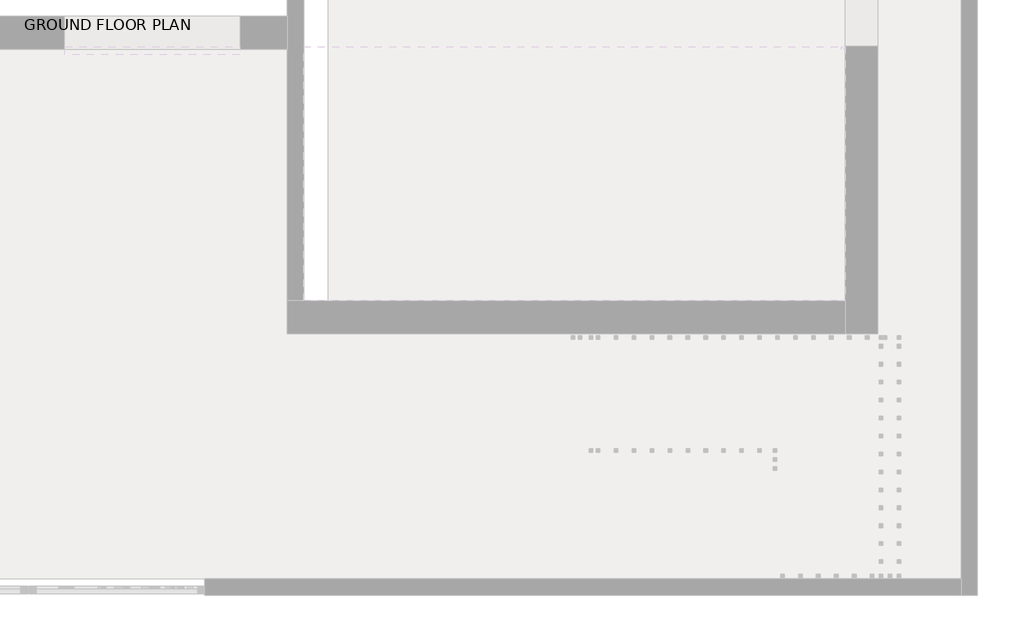
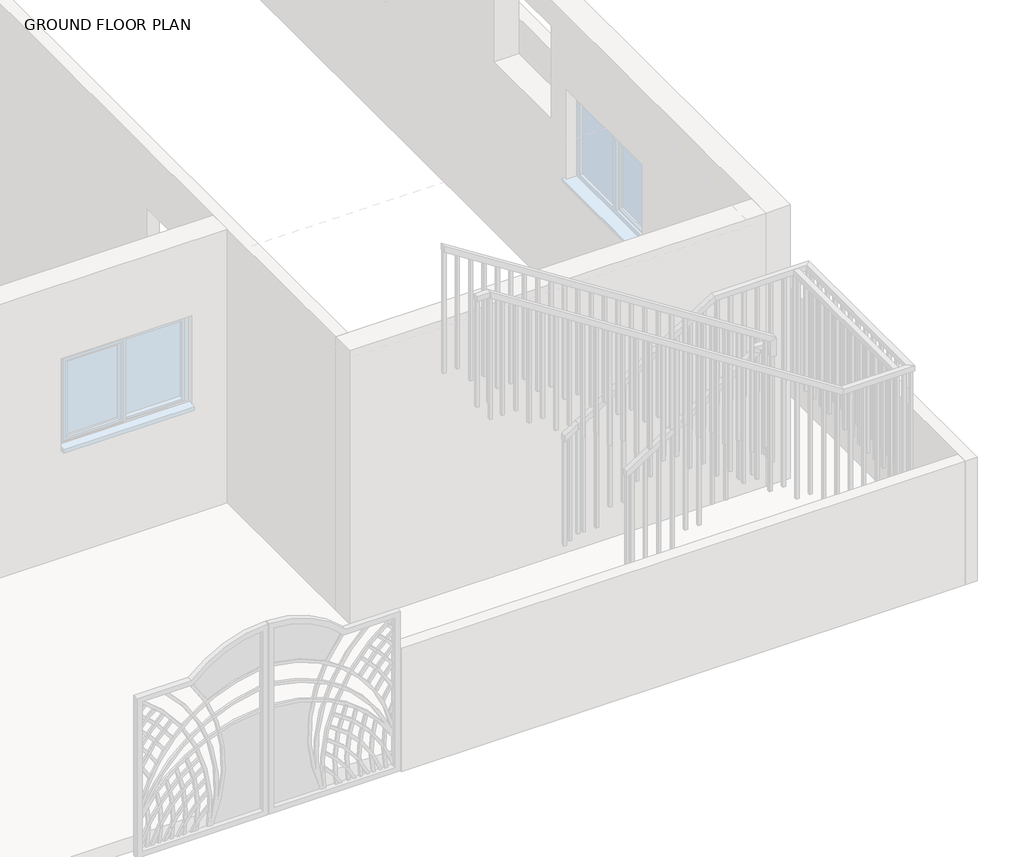
# One storey, part 7 of 23: 2 railings.
"""IFC4 building model written with IfcOpenShell, lengths in millimetres."""

from ifc_helpers import new_model, si_unit, frame, origin, place, context, project, spatial, polyline, outline, extrude, faceted_brep, element, save

model = new_model("IFC4")

# Units and contexts
model_context = context("Model", 3, world=origin())
ifc_project = project(units=[si_unit("LENGTHUNIT", "METRE", prefix="MILLI")], contexts=[model_context])

# Site, building, storey
site = spatial("IfcSite", under=ifc_project)
building = spatial("IfcBuilding", under=site)
storey = spatial("IfcBuildingStorey", under=building, Name="GROUND FLOOR PLAN", Elevation=487.68)

# Railings
placement = place(None, origin())
element("IfcRailing", 1, ObjectType="1100mm", at=placement, inside=storey, context=model_context, shape_type="SolidModel", body=[
    faceted_brep([(-8680.149573, -11007.9255223, 1912.8), (-8680.149573, -11007.9255223, 1853.4423995), (-8680.149573, -11057.9255223, 1853.4423995), (-8680.149573, -11057.9255223, 1912.8), (-7484.3306254, -11007.9255223, 2677.8717446), (-7434.3306254, -11007.9255223, 2650.5035914), (-7434.3306254, -11057.9255223, 2650.5035914), (-7484.3306254, -11057.9255223, 2677.8717446), (-7484.3306254, -11007.9255223, 2725.6), (-7434.3306254, -11007.9255223, 2675.6), (-7434.3306254, -11057.9255223, 2675.6), (-7484.3306254, -11057.9255223, 2725.6), (-7359.3306254, -11007.9255223, 2725.6), (-7359.3306254, -11007.9255223, 2675.6), (-7409.3306254, -11057.9255223, 2675.6), (-7409.3306254, -11057.9255223, 2725.6), (-7359.3306254, -11132.9255223, 2725.6), (-7359.3306254, -11132.9255223, 2675.6), (-7409.3306254, -11132.9255223, 2675.6), (-7409.3306254, -11132.9255223, 2725.6), (-7359.3306254, -11134.9255223, 2725.6), (-7409.3306254, -11134.9255223, 2725.6), (-7409.3306254, -11184.9255223, 2675.6), (-7359.3306254, -11184.9255223, 2675.6)], [[[0, 1, 2, 3]], [[1, 0, 4, 5]], [[2, 1, 5, 6]], [[3, 2, 6, 7]], [[0, 3, 7, 4]], [[5, 4, 8, 9]], [[6, 5, 9, 10]], [[7, 6, 10, 11]], [[4, 7, 11, 8]], [[9, 8, 12, 13]], [[10, 9, 13, 14]], [[11, 10, 14, 15]], [[8, 11, 15, 12]], [[13, 12, 16, 17]], [[14, 13, 17, 18]], [[15, 14, 18, 19]], [[12, 15, 19, 16]], [[20, 21, 22, 23]], [[17, 16, 20, 23]], [[18, 17, 23, 22]], [[19, 18, 22, 21]], [[16, 19, 21, 20]]]),
    faceted_brep([(-7359.3306254, -11184.9255223, 2855.9055527), (-7409.3306254, -11184.9255223, 2828.5415543), (-7409.3306254, -11134.9255223, 2828.5415543), (-7359.3306254, -11134.9255223, 2855.9055527), (-10457.8773536, -11184.9255223, 4838.88), (-10457.8773536, -11134.9255223, 4838.88), (-10457.8773536, -11134.9255223, 4779.517542), (-10457.8773536, -11184.9255223, 4779.517542)], [[[0, 1, 2, 3]], [[4, 5, 6, 7]], [[1, 0, 4, 7]], [[2, 1, 7, 6]], [[3, 2, 6, 5]], [[0, 3, 5, 4]]]),
    faceted_brep([(-7359.3306254, -11134.9255223, 2725.6), (-7359.3306254, -11184.9255223, 2675.6), (-7409.3306254, -11184.9255223, 2675.6), (-7409.3306254, -11134.9255223, 2725.6), (-7359.3306254, -11134.9255223, 2855.9055527), (-7409.3306254, -11134.9255223, 2828.5415543), (-7409.3306254, -11184.9255223, 2828.5415543), (-7359.3306254, -11184.9255223, 2855.9055527)], [[[0, 1, 2, 3]], [[4, 5, 6, 7]], [[1, 0, 4, 7]], [[2, 1, 7, 6]], [[3, 2, 6, 5]], [[0, 3, 5, 4]]]),
    extrude(outline(polyline([(3576.32, -10434.3306254), (4764.4483614, -10434.3306254), (4780.4475912, -10459.3306254), (3576.32, -10459.3306254), (3576.32, -10434.3306254)])), frame((0.0, -11172.4255223, 0.0), z_axis=(0.0, 1.0, 0.0), x_axis=(0.0, 0.0, 1.0)), (0.0, 0.0, 1.0), 25.0),
    extrude(outline(polyline([(3576.32, -10309.3306254), (4684.4522123, -10309.3306254), (4700.4514422, -10334.3306254), (3576.32, -10334.3306254), (3576.32, -10309.3306254)])), frame((0.0, -11172.4255223, 0.0), z_axis=(0.0, 1.0, 0.0), x_axis=(0.0, 0.0, 1.0)), (0.0, 0.0, 1.0), 25.0),
    extrude(outline(polyline([(3413.76, -10184.3306254), (4604.4560633, -10184.3306254), (4620.4552931, -10209.3306254), (3413.76, -10209.3306254), (3413.76, -10184.3306254)])), frame((0.0, -11172.4255223, 0.0), z_axis=(0.0, 1.0, 0.0), x_axis=(0.0, 0.0, 1.0)), (0.0, 0.0, 1.0), 25.0),
    extrude(outline(polyline([(3413.76, -10059.3306254), (4524.4599142, -10059.3306254), (4540.459144, -10084.3306254), (3413.76, -10084.3306254), (3413.76, -10059.3306254)])), frame((0.0, -11172.4255223, 0.0), z_axis=(0.0, 1.0, 0.0), x_axis=(0.0, 0.0, 1.0)), (0.0, 0.0, 1.0), 25.0),
    extrude(outline(polyline([(3251.2, -9934.3306254), (4444.4637652, -9934.3306254), (4460.462995, -9959.3306254), (3251.2, -9959.3306254), (3251.2, -9934.3306254)])), frame((0.0, -11172.4255223, 0.0), z_axis=(0.0, 1.0, 0.0), x_axis=(0.0, 0.0, 1.0)), (0.0, 0.0, 1.0), 25.0),
    extrude(outline(polyline([(3251.2, -9809.3306254), (4364.4676161, -9809.3306254), (4380.4668459, -9834.3306254), (3251.2, -9834.3306254), (3251.2, -9809.3306254)])), frame((0.0, -11172.4255223, 0.0), z_axis=(0.0, 1.0, 0.0), x_axis=(0.0, 0.0, 1.0)), (0.0, 0.0, 1.0), 25.0),
    extrude(outline(polyline([(3251.2, -9684.3306254), (4284.4714671, -9684.3306254), (4300.4706969, -9709.3306254), (3251.2, -9709.3306254), (3251.2, -9684.3306254)])), frame((0.0, -11172.4255223, 0.0), z_axis=(0.0, 1.0, 0.0), x_axis=(0.0, 0.0, 1.0)), (0.0, 0.0, 1.0), 25.0),
    extrude(outline(polyline([(3088.64, -9559.3306254), (4204.475318, -9559.3306254), (4220.4745478, -9584.3306254), (3088.64, -9584.3306254), (3088.64, -9559.3306254)])), frame((0.0, -11172.4255223, 0.0), z_axis=(0.0, 1.0, 0.0), x_axis=(0.0, 0.0, 1.0)), (0.0, 0.0, 1.0), 25.0),
    extrude(outline(polyline([(3088.64, -9434.3306254), (4124.479169, -9434.3306254), (4140.4783988, -9459.3306254), (3088.64, -9459.3306254), (3088.64, -9434.3306254)])), frame((0.0, -11172.4255223, 0.0), z_axis=(0.0, 1.0, 0.0), x_axis=(0.0, 0.0, 1.0)), (0.0, 0.0, 1.0), 25.0),
    extrude(outline(polyline([(2926.08, -9309.3306254), (4044.4830199, -9309.3306254), (4060.4822497, -9334.3306254), (2926.08, -9334.3306254), (2926.08, -9309.3306254)])), frame((0.0, -11172.4255223, 0.0), z_axis=(0.0, 1.0, 0.0), x_axis=(0.0, 0.0, 1.0)), (0.0, 0.0, 1.0), 25.0),
    extrude(outline(polyline([(2926.08, -9184.3306254), (3964.4868709, -9184.3306254), (3980.4861007, -9209.3306254), (2926.08, -9209.3306254), (2926.08, -9184.3306254)])), frame((0.0, -11172.4255223, 0.0), z_axis=(0.0, 1.0, 0.0), x_axis=(0.0, 0.0, 1.0)), (0.0, 0.0, 1.0), 25.0),
    extrude(outline(polyline([(2763.52, -9059.3306254), (3884.4907218, -9059.3306254), (3900.4899516, -9084.3306254), (2763.52, -9084.3306254), (2763.52, -9059.3306254)])), frame((0.0, -11172.4255223, 0.0), z_axis=(0.0, 1.0, 0.0), x_axis=(0.0, 0.0, 1.0)), (0.0, 0.0, 1.0), 25.0),
    extrude(outline(polyline([(2763.52, -8934.3306254), (3804.4945728, -8934.3306254), (3820.4938026, -8959.3306254), (2763.52, -8959.3306254), (2763.52, -8934.3306254)])), frame((0.0, -11172.4255223, 0.0), z_axis=(0.0, 1.0, 0.0), x_axis=(0.0, 0.0, 1.0)), (0.0, 0.0, 1.0), 25.0),
    extrude(outline(polyline([(2600.96, -8809.3306254), (3724.4984237, -8809.3306254), (3740.4976535, -8834.3306254), (2600.96, -8834.3306254), (2600.96, -8809.3306254)])), frame((0.0, -11172.4255223, 0.0), z_axis=(0.0, 1.0, 0.0), x_axis=(0.0, 0.0, 1.0)), (0.0, 0.0, 1.0), 25.0),
    extrude(outline(polyline([(2600.96, -8684.3306254), (3644.5022747, -8684.3306254), (3660.5015045, -8709.3306254), (2600.96, -8709.3306254), (2600.96, -8684.3306254)])), frame((0.0, -11172.4255223, 0.0), z_axis=(0.0, 1.0, 0.0), x_axis=(0.0, 0.0, 1.0)), (0.0, 0.0, 1.0), 25.0),
    extrude(outline(polyline([(2438.4, -8559.3306254), (3564.5061256, -8559.3306254), (3580.5053554, -8584.3306254), (2438.4, -8584.3306254), (2438.4, -8559.3306254)])), frame((0.0, -11172.4255223, 0.0), z_axis=(0.0, 1.0, 0.0), x_axis=(0.0, 0.0, 1.0)), (0.0, 0.0, 1.0), 25.0),
    extrude(outline(polyline([(2438.4, -8434.3306254), (3484.5099766, -8434.3306254), (3500.5092064, -8459.3306254), (2438.4, -8459.3306254), (2438.4, -8434.3306254)])), frame((0.0, -11172.4255223, 0.0), z_axis=(0.0, 1.0, 0.0), x_axis=(0.0, 0.0, 1.0)), (0.0, 0.0, 1.0), 25.0),
    extrude(outline(polyline([(2275.84, -8309.3306254), (3404.5138275, -8309.3306254), (3420.5130573, -8334.3306254), (2275.84, -8334.3306254), (2275.84, -8309.3306254)])), frame((0.0, -11172.4255223, 0.0), z_axis=(0.0, 1.0, 0.0), x_axis=(0.0, 0.0, 1.0)), (0.0, 0.0, 1.0), 25.0),
    extrude(outline(polyline([(2275.84, -8184.3306254), (3324.5176785, -8184.3306254), (3340.5169083, -8209.3306254), (2275.84, -8209.3306254), (2275.84, -8184.3306254)])), frame((0.0, -11172.4255223, 0.0), z_axis=(0.0, 1.0, 0.0), x_axis=(0.0, 0.0, 1.0)), (0.0, 0.0, 1.0), 25.0),
    extrude(outline(polyline([(2113.28, -8059.3306254), (3244.5215294, -8059.3306254), (3260.5207592, -8084.3306254), (2113.28, -8084.3306254), (2113.28, -8059.3306254)])), frame((0.0, -11172.4255223, 0.0), z_axis=(0.0, 1.0, 0.0), x_axis=(0.0, 0.0, 1.0)), (0.0, 0.0, 1.0), 25.0),
    extrude(outline(polyline([(2113.28, -7934.3306254), (3164.5253804, -7934.3306254), (3180.5246102, -7959.3306254), (2113.28, -7959.3306254), (2113.28, -7934.3306254)])), frame((0.0, -11172.4255223, 0.0), z_axis=(0.0, 1.0, 0.0), x_axis=(0.0, 0.0, 1.0)), (0.0, 0.0, 1.0), 25.0),
    extrude(outline(polyline([(1950.72, -7809.3306254), (3084.5292313, -7809.3306254), (3100.5284611, -7834.3306254), (1950.72, -7834.3306254), (1950.72, -7809.3306254)])), frame((0.0, -11172.4255223, 0.0), z_axis=(0.0, 1.0, 0.0), x_axis=(0.0, 0.0, 1.0)), (0.0, 0.0, 1.0), 25.0),
    extrude(outline(polyline([(1950.72, -7684.3306254), (3004.5330823, -7684.3306254), (3020.5323121, -7709.3306254), (1950.72, -7709.3306254), (1950.72, -7684.3306254)])), frame((0.0, -11172.4255223, 0.0), z_axis=(0.0, 1.0, 0.0), x_axis=(0.0, 0.0, 1.0)), (0.0, 0.0, 1.0), 25.0),
    extrude(outline(polyline([(1788.16, -7559.3306254), (2924.5369332, -7559.3306254), (2940.536163, -7584.3306254), (1788.16, -7584.3306254), (1788.16, -7559.3306254)])), frame((0.0, -11172.4255223, 0.0), z_axis=(0.0, 1.0, 0.0), x_axis=(0.0, 0.0, 1.0)), (0.0, 0.0, 1.0), 25.0),
    extrude(outline(polyline([(1788.16, -7434.3306254), (2844.5407841, -7434.3306254), (2860.540014, -7459.3306254), (1788.16, -7459.3306254), (1788.16, -7434.3306254)])), frame((0.0, -11172.4255223, 0.0), z_axis=(0.0, 1.0, 0.0), x_axis=(0.0, 0.0, 1.0)), (0.0, 0.0, 1.0), 25.0),
    extrude(outline(polyline([(-7396.8306254, -11082.9255223), (-7371.8306254, -11082.9255223), (-7371.8306254, -11107.9255223), (-7396.8306254, -11107.9255223), (-7396.8306254, -11082.9255223)])), frame((0.0, 0.0, 1625.6), z_axis=(0.0, 0.0, 1.0), x_axis=(1.0, 0.0, 0.0)), (0.0, 0.0, 1.0), 1050.0),
    extrude(outline(polyline([(2605.1944115, -7505.149573), (1463.04, -7505.149573), (1463.04, -7480.149573), (2621.1891352, -7480.149573), (2605.1944115, -7505.149573)])), frame((0.0, -11045.4255223, 0.0), z_axis=(0.0, 1.0, 0.0), x_axis=(0.0, 0.0, 1.0)), (0.0, 0.0, 1.0), 25.0),
    extrude(outline(polyline([(2525.2207932, -7630.149573), (1463.04, -7630.149573), (1463.04, -7605.149573), (2541.2155169, -7605.149573), (2525.2207932, -7630.149573)])), frame((0.0, -11045.4255223, 0.0), z_axis=(0.0, 1.0, 0.0), x_axis=(0.0, 0.0, 1.0)), (0.0, 0.0, 1.0), 25.0),
    extrude(outline(polyline([(2445.2471749, -7755.149573), (1300.48, -7755.149573), (1300.48, -7730.149573), (2461.2418986, -7730.149573), (2445.2471749, -7755.149573)])), frame((0.0, -11045.4255223, 0.0), z_axis=(0.0, 1.0, 0.0), x_axis=(0.0, 0.0, 1.0)), (0.0, 0.0, 1.0), 25.0),
    extrude(outline(polyline([(2365.2735566, -7880.149573), (1300.48, -7880.149573), (1300.48, -7855.149573), (2381.2682803, -7855.149573), (2365.2735566, -7880.149573)])), frame((0.0, -11045.4255223, 0.0), z_axis=(0.0, 1.0, 0.0), x_axis=(0.0, 0.0, 1.0)), (0.0, 0.0, 1.0), 25.0),
    extrude(outline(polyline([(2285.2999383, -8005.149573), (1137.92, -8005.149573), (1137.92, -7980.149573), (2301.294662, -7980.149573), (2285.2999383, -8005.149573)])), frame((0.0, -11045.4255223, 0.0), z_axis=(0.0, 1.0, 0.0), x_axis=(0.0, 0.0, 1.0)), (0.0, 0.0, 1.0), 25.0),
    extrude(outline(polyline([(2205.32632, -8130.149573), (1137.92, -8130.149573), (1137.92, -8105.149573), (2221.3210437, -8105.149573), (2205.32632, -8130.149573)])), frame((0.0, -11045.4255223, 0.0), z_axis=(0.0, 1.0, 0.0), x_axis=(0.0, 0.0, 1.0)), (0.0, 0.0, 1.0), 25.0),
    extrude(outline(polyline([(2125.3527017, -8255.149573), (975.36, -8255.149573), (975.36, -8230.149573), (2141.3474254, -8230.149573), (2125.3527017, -8255.149573)])), frame((0.0, -11045.4255223, 0.0), z_axis=(0.0, 1.0, 0.0), x_axis=(0.0, 0.0, 1.0)), (0.0, 0.0, 1.0), 25.0),
    extrude(outline(polyline([(2045.3790834, -8380.149573), (975.36, -8380.149573), (975.36, -8355.149573), (2061.3738071, -8355.149573), (2045.3790834, -8380.149573)])), frame((0.0, -11045.4255223, 0.0), z_axis=(0.0, 1.0, 0.0), x_axis=(0.0, 0.0, 1.0)), (0.0, 0.0, 1.0), 25.0),
    extrude(outline(polyline([(1965.4054651, -8505.149573), (812.8, -8505.149573), (812.8, -8480.149573), (1981.4001888, -8480.149573), (1965.4054651, -8505.149573)])), frame((0.0, -11045.4255223, 0.0), z_axis=(0.0, 1.0, 0.0), x_axis=(0.0, 0.0, 1.0)), (0.0, 0.0, 1.0), 25.0),
    extrude(outline(polyline([(1885.4318468, -8630.149573), (812.8, -8630.149573), (812.8, -8605.149573), (1901.4265705, -8605.149573), (1885.4318468, -8630.149573)])), frame((0.0, -11045.4255223, 0.0), z_axis=(0.0, 1.0, 0.0), x_axis=(0.0, 0.0, 1.0)), (0.0, 0.0, 1.0), 25.0),
    extrude(outline(polyline([(-7396.8306254, -11147.4255223), (-7371.8306254, -11147.4255223), (-7371.8306254, -11172.4255223), (-7396.8306254, -11172.4255223), (-7396.8306254, -11147.4255223)])), frame((0.0, 0.0, 1625.6), z_axis=(0.0, 0.0, 1.0), x_axis=(1.0, 0.0, 0.0)), (0.0, 0.0, 1.0), 1050.0),
    extrude(outline(polyline([(-7396.8306254, -11045.4255223), (-7396.8306254, -11020.4255223), (-7371.8306254, -11020.4255223), (-7371.8306254, -11045.4255223), (-7396.8306254, -11045.4255223)])), frame((0.0, 0.0, 1625.6), z_axis=(0.0, 0.0, 1.0), x_axis=(1.0, 0.0, 0.0)), (0.0, 0.0, 1.0), 1050.0),
    extrude(outline(polyline([(3576.32, -10432.8773536), (4763.5183122, -10432.8773536), (4779.517542, -10457.8773536), (3576.32, -10457.8773536), (3576.32, -10432.8773536)])), frame((0.0, -11172.4255223, 0.0), z_axis=(0.0, 1.0, 0.0), x_axis=(0.0, 0.0, 1.0)), (0.0, 0.0, 1.0), 25.0),
    extrude(outline(polyline([(1853.4423995, -8680.149573), (812.8, -8680.149573), (812.8, -8655.149573), (1869.4371231, -8655.149573), (1853.4423995, -8680.149573)])), frame((0.0, -11045.4255223, 0.0), z_axis=(0.0, 1.0, 0.0), x_axis=(0.0, 0.0, 1.0)), (0.0, 0.0, 1.0), 25.0),
])
element("IfcRailing", 2, ObjectType="1100mm", at=placement, inside=storey, context=model_context, shape_type="SolidModel", body=[
    faceted_brep([(-8680.149573, -10220.0521308, 1912.8), (-8680.149573, -10220.0521308, 1853.4423995), (-8680.149573, -10270.0521308, 1853.4423995), (-8680.149573, -10270.0521308, 1912.8), (-7409.7306254, -10220.0521308, 2725.6), (-7395.1045513, -10220.0521308, 2675.6), (-7395.1045513, -10270.0521308, 2675.6), (-7409.7306254, -10270.0521308, 2725.6), (-6495.8132565, -10220.0521308, 2725.6), (-6495.8132565, -10220.0521308, 2675.6), (-6545.8132565, -10270.0521308, 2675.6), (-6545.8132565, -10270.0521308, 2725.6), (-6495.8132565, -11933.6860066, 2725.6), (-6495.8132565, -11933.6860066, 2675.6), (-6545.8132565, -11883.6860066, 2675.6), (-6545.8132565, -11883.6860066, 2725.6), (-7155.718398, -11933.6860066, 2725.6), (-7170.3479429, -11933.6860066, 2675.6), (-7170.3479429, -11883.6860066, 2675.6), (-7155.718398, -11883.6860066, 2725.6), (-10457.8773536, -11933.6860066, 4838.88), (-10457.8773536, -11883.6860066, 4838.88), (-10457.8773536, -11883.6860066, 4779.517542), (-10457.8773536, -11933.6860066, 4779.517542)], [[[0, 1, 2, 3]], [[1, 0, 4, 5]], [[2, 1, 5, 6]], [[3, 2, 6, 7]], [[0, 3, 7, 4]], [[5, 4, 8, 9]], [[6, 5, 9, 10]], [[7, 6, 10, 11]], [[4, 7, 11, 8]], [[9, 8, 12, 13]], [[10, 9, 13, 14]], [[11, 10, 14, 15]], [[8, 11, 15, 12]], [[13, 12, 16, 17]], [[14, 13, 17, 18]], [[15, 14, 18, 19]], [[12, 15, 19, 16]], [[20, 21, 22, 23]], [[17, 16, 20, 23]], [[18, 17, 23, 22]], [[19, 18, 22, 21]], [[16, 19, 21, 20]]]),
    extrude(outline(polyline([(4691.8007425, -10320.8132565), (4707.7999723, -10345.8132565), (3576.32, -10345.8132565), (3576.32, -10320.8132565), (4691.8007425, -10320.8132565)])), frame((0.0, -11921.1860066, 0.0), z_axis=(0.0, 1.0, 0.0), x_axis=(0.0, 0.0, 1.0)), (0.0, 0.0, 1.0), 25.0),
    extrude(outline(polyline([(4611.8045935, -10195.8132565), (4627.8038233, -10220.8132565), (3576.32, -10220.8132565), (3576.32, -10195.8132565), (4611.8045935, -10195.8132565)])), frame((0.0, -11921.1860066, 0.0), z_axis=(0.0, 1.0, 0.0), x_axis=(0.0, 0.0, 1.0)), (0.0, 0.0, 1.0), 25.0),
    extrude(outline(polyline([(4531.8084444, -10070.8132565), (4547.8076742, -10095.8132565), (3413.76, -10095.8132565), (3413.76, -10070.8132565), (4531.8084444, -10070.8132565)])), frame((0.0, -11921.1860066, 0.0), z_axis=(0.0, 1.0, 0.0), x_axis=(0.0, 0.0, 1.0)), (0.0, 0.0, 1.0), 25.0),
    extrude(outline(polyline([(4451.8122954, -9945.8132565), (4467.8115252, -9970.8132565), (3413.76, -9970.8132565), (3413.76, -9945.8132565), (4451.8122954, -9945.8132565)])), frame((0.0, -11921.1860066, 0.0), z_axis=(0.0, 1.0, 0.0), x_axis=(0.0, 0.0, 1.0)), (0.0, 0.0, 1.0), 25.0),
    extrude(outline(polyline([(4371.8161463, -9820.8132565), (4387.8153761, -9845.8132565), (3251.2, -9845.8132565), (3251.2, -9820.8132565), (4371.8161463, -9820.8132565)])), frame((0.0, -11921.1860066, 0.0), z_axis=(0.0, 1.0, 0.0), x_axis=(0.0, 0.0, 1.0)), (0.0, 0.0, 1.0), 25.0),
    extrude(outline(polyline([(4291.8423995, -9695.8132565), (4307.8371231, -9720.8132565), (3251.2, -9720.8132565), (3251.2, -9695.8132565), (4291.8423995, -9695.8132565)])), frame((0.0, -11921.1860066, 0.0), z_axis=(0.0, 1.0, 0.0), x_axis=(0.0, 0.0, 1.0)), (0.0, 0.0, 1.0), 25.0),
    extrude(outline(polyline([(4211.8238482, -9570.8132565), (4227.823078, -9595.8132565), (3088.64, -9595.8132565), (3088.64, -9570.8132565), (4211.8238482, -9570.8132565)])), frame((0.0, -11921.1860066, 0.0), z_axis=(0.0, 1.0, 0.0), x_axis=(0.0, 0.0, 1.0)), (0.0, 0.0, 1.0), 25.0),
    extrude(outline(polyline([(4131.8276992, -9445.8132565), (4147.826929, -9470.8132565), (3088.64, -9470.8132565), (3088.64, -9445.8132565), (4131.8276992, -9445.8132565)])), frame((0.0, -11921.1860066, 0.0), z_axis=(0.0, 1.0, 0.0), x_axis=(0.0, 0.0, 1.0)), (0.0, 0.0, 1.0), 25.0),
    extrude(outline(polyline([(4051.8315501, -9320.8132565), (4067.8307799, -9345.8132565), (2926.08, -9345.8132565), (2926.08, -9320.8132565), (4051.8315501, -9320.8132565)])), frame((0.0, -11921.1860066, 0.0), z_axis=(0.0, 1.0, 0.0), x_axis=(0.0, 0.0, 1.0)), (0.0, 0.0, 1.0), 25.0),
    extrude(outline(polyline([(3971.835401, -9195.8132565), (3987.8346309, -9220.8132565), (2926.08, -9220.8132565), (2926.08, -9195.8132565), (3971.835401, -9195.8132565)])), frame((0.0, -11921.1860066, 0.0), z_axis=(0.0, 1.0, 0.0), x_axis=(0.0, 0.0, 1.0)), (0.0, 0.0, 1.0), 25.0),
    extrude(outline(polyline([(3891.839252, -9070.8132565), (3907.8384818, -9095.8132565), (2763.52, -9095.8132565), (2763.52, -9070.8132565), (3891.839252, -9070.8132565)])), frame((0.0, -11921.1860066, 0.0), z_axis=(0.0, 1.0, 0.0), x_axis=(0.0, 0.0, 1.0)), (0.0, 0.0, 1.0), 25.0),
    extrude(outline(polyline([(3811.8431029, -8945.8132565), (3827.8423328, -8970.8132565), (2763.52, -8970.8132565), (2763.52, -8945.8132565), (3811.8431029, -8945.8132565)])), frame((0.0, -11921.1860066, 0.0), z_axis=(0.0, 1.0, 0.0), x_axis=(0.0, 0.0, 1.0)), (0.0, 0.0, 1.0), 25.0),
    extrude(outline(polyline([(3731.8469539, -8820.8132565), (3747.8461837, -8845.8132565), (2600.96, -8845.8132565), (2600.96, -8820.8132565), (3731.8469539, -8820.8132565)])), frame((0.0, -11921.1860066, 0.0), z_axis=(0.0, 1.0, 0.0), x_axis=(0.0, 0.0, 1.0)), (0.0, 0.0, 1.0), 25.0),
    extrude(outline(polyline([(3651.8508048, -8695.8132565), (3667.8500347, -8720.8132565), (2600.96, -8720.8132565), (2600.96, -8695.8132565), (3651.8508048, -8695.8132565)])), frame((0.0, -11921.1860066, 0.0), z_axis=(0.0, 1.0, 0.0), x_axis=(0.0, 0.0, 1.0)), (0.0, 0.0, 1.0), 25.0),
    extrude(outline(polyline([(3571.8546558, -8570.8132565), (3587.8538856, -8595.8132565), (2438.4, -8595.8132565), (2438.4, -8570.8132565), (3571.8546558, -8570.8132565)])), frame((0.0, -11921.1860066, 0.0), z_axis=(0.0, 1.0, 0.0), x_axis=(0.0, 0.0, 1.0)), (0.0, 0.0, 1.0), 25.0),
    extrude(outline(polyline([(3491.8585067, -8445.8132565), (3507.8577365, -8470.8132565), (2438.4, -8470.8132565), (2438.4, -8445.8132565), (3491.8585067, -8445.8132565)])), frame((0.0, -11921.1860066, 0.0), z_axis=(0.0, 1.0, 0.0), x_axis=(0.0, 0.0, 1.0)), (0.0, 0.0, 1.0), 25.0),
    extrude(outline(polyline([(3411.8623577, -8320.8132565), (3427.8615875, -8345.8132565), (2275.84, -8345.8132565), (2275.84, -8320.8132565), (3411.8623577, -8320.8132565)])), frame((0.0, -11921.1860066, 0.0), z_axis=(0.0, 1.0, 0.0), x_axis=(0.0, 0.0, 1.0)), (0.0, 0.0, 1.0), 25.0),
    extrude(outline(polyline([(3331.8662086, -8195.8132565), (3347.8654384, -8220.8132565), (2275.84, -8220.8132565), (2275.84, -8195.8132565), (3331.8662086, -8195.8132565)])), frame((0.0, -11921.1860066, 0.0), z_axis=(0.0, 1.0, 0.0), x_axis=(0.0, 0.0, 1.0)), (0.0, 0.0, 1.0), 25.0),
    extrude(outline(polyline([(3251.8700596, -8070.8132565), (3267.8692894, -8095.8132565), (2113.28, -8095.8132565), (2113.28, -8070.8132565), (3251.8700596, -8070.8132565)])), frame((0.0, -11921.1860066, 0.0), z_axis=(0.0, 1.0, 0.0), x_axis=(0.0, 0.0, 1.0)), (0.0, 0.0, 1.0), 25.0),
    extrude(outline(polyline([(3171.8739105, -7945.8132565), (3187.8731403, -7970.8132565), (2113.28, -7970.8132565), (2113.28, -7945.8132565), (3171.8739105, -7945.8132565)])), frame((0.0, -11921.1860066, 0.0), z_axis=(0.0, 1.0, 0.0), x_axis=(0.0, 0.0, 1.0)), (0.0, 0.0, 1.0), 25.0),
    extrude(outline(polyline([(3091.8777615, -7820.8132565), (3107.8769913, -7845.8132565), (1950.72, -7845.8132565), (1950.72, -7820.8132565), (3091.8777615, -7820.8132565)])), frame((0.0, -11921.1860066, 0.0), z_axis=(0.0, 1.0, 0.0), x_axis=(0.0, 0.0, 1.0)), (0.0, 0.0, 1.0), 25.0),
    extrude(outline(polyline([(3011.8816124, -7695.8132565), (3027.8808422, -7720.8132565), (1950.72, -7720.8132565), (1950.72, -7695.8132565), (3011.8816124, -7695.8132565)])), frame((0.0, -11921.1860066, 0.0), z_axis=(0.0, 1.0, 0.0), x_axis=(0.0, 0.0, 1.0)), (0.0, 0.0, 1.0), 25.0),
    extrude(outline(polyline([(2931.8854634, -7570.8132565), (2947.8846932, -7595.8132565), (1788.16, -7595.8132565), (1788.16, -7570.8132565), (2931.8854634, -7570.8132565)])), frame((0.0, -11921.1860066, 0.0), z_axis=(0.0, 1.0, 0.0), x_axis=(0.0, 0.0, 1.0)), (0.0, 0.0, 1.0), 25.0),
    extrude(outline(polyline([(2851.8893143, -7445.8132565), (2867.8885441, -7470.8132565), (1788.16, -7470.8132565), (1788.16, -7445.8132565), (2851.8893143, -7445.8132565)])), frame((0.0, -11921.1860066, 0.0), z_axis=(0.0, 1.0, 0.0), x_axis=(0.0, 0.0, 1.0)), (0.0, 0.0, 1.0), 25.0),
    extrude(outline(polyline([(2771.8931653, -7320.8132565), (2787.8923951, -7345.8132565), (1625.6, -7345.8132565), (1625.6, -7320.8132565), (2771.8931653, -7320.8132565)])), frame((0.0, -11921.1860066, 0.0), z_axis=(0.0, 1.0, 0.0), x_axis=(0.0, 0.0, 1.0)), (0.0, 0.0, 1.0), 25.0),
    extrude(outline(polyline([(2691.8970162, -7195.8132565), (2707.896246, -7220.8132565), (1625.6, -7220.8132565), (1625.6, -7195.8132565), (2691.8970162, -7195.8132565)])), frame((0.0, -11921.1860066, 0.0), z_axis=(0.0, 1.0, 0.0), x_axis=(0.0, 0.0, 1.0)), (0.0, 0.0, 1.0), 25.0),
    extrude(outline(polyline([(-7070.8132565, -11921.1860066), (-7095.8132565, -11921.1860066), (-7095.8132565, -11896.1860066), (-7070.8132565, -11896.1860066), (-7070.8132565, -11921.1860066)])), frame((0.0, 0.0, 1625.6), z_axis=(0.0, 0.0, 1.0), x_axis=(1.0, 0.0, 0.0)), (0.0, 0.0, 1.0), 1050.0),
    extrude(outline(polyline([(-6945.8132565, -11921.1860066), (-6970.8132565, -11921.1860066), (-6970.8132565, -11896.1860066), (-6945.8132565, -11896.1860066), (-6945.8132565, -11921.1860066)])), frame((0.0, 0.0, 1625.6), z_axis=(0.0, 0.0, 1.0), x_axis=(1.0, 0.0, 0.0)), (0.0, 0.0, 1.0), 1050.0),
    extrude(outline(polyline([(-6820.8132565, -11921.1860066), (-6845.8132565, -11921.1860066), (-6845.8132565, -11896.1860066), (-6820.8132565, -11896.1860066), (-6820.8132565, -11921.1860066)])), frame((0.0, 0.0, 1625.6), z_axis=(0.0, 0.0, 1.0), x_axis=(1.0, 0.0, 0.0)), (0.0, 0.0, 1.0), 1050.0),
    extrude(outline(polyline([(-6695.8132565, -11921.1860066), (-6720.8132565, -11921.1860066), (-6720.8132565, -11896.1860066), (-6695.8132565, -11896.1860066), (-6695.8132565, -11921.1860066)])), frame((0.0, 0.0, 1625.6), z_axis=(0.0, 0.0, 1.0), x_axis=(1.0, 0.0, 0.0)), (0.0, 0.0, 1.0), 1050.0),
    extrude(outline(polyline([(-6570.8132565, -11921.1860066), (-6595.8132565, -11921.1860066), (-6595.8132565, -11896.1860066), (-6570.8132565, -11896.1860066), (-6570.8132565, -11921.1860066)])), frame((0.0, 0.0, 1625.6), z_axis=(0.0, 0.0, 1.0), x_axis=(1.0, 0.0, 0.0)), (0.0, 0.0, 1.0), 1050.0),
    extrude(outline(polyline([(-6508.3132565, -11795.0521308), (-6508.3132565, -11820.0521308), (-6533.3132565, -11820.0521308), (-6533.3132565, -11795.0521308), (-6508.3132565, -11795.0521308)])), frame((0.0, 0.0, 1625.6), z_axis=(0.0, 0.0, 1.0), x_axis=(1.0, 0.0, 0.0)), (0.0, 0.0, 1.0), 1050.0),
    extrude(outline(polyline([(-6508.3132565, -11670.0521308), (-6508.3132565, -11695.0521308), (-6533.3132565, -11695.0521308), (-6533.3132565, -11670.0521308), (-6508.3132565, -11670.0521308)])), frame((0.0, 0.0, 1625.6), z_axis=(0.0, 0.0, 1.0), x_axis=(1.0, 0.0, 0.0)), (0.0, 0.0, 1.0), 1050.0),
    extrude(outline(polyline([(-6508.3132565, -11545.0521308), (-6508.3132565, -11570.0521308), (-6533.3132565, -11570.0521308), (-6533.3132565, -11545.0521308), (-6508.3132565, -11545.0521308)])), frame((0.0, 0.0, 1625.6), z_axis=(0.0, 0.0, 1.0), x_axis=(1.0, 0.0, 0.0)), (0.0, 0.0, 1.0), 1050.0),
    extrude(outline(polyline([(-6508.3132565, -11420.0521308), (-6508.3132565, -11445.0521308), (-6533.3132565, -11445.0521308), (-6533.3132565, -11420.0521308), (-6508.3132565, -11420.0521308)])), frame((0.0, 0.0, 1625.6), z_axis=(0.0, 0.0, 1.0), x_axis=(1.0, 0.0, 0.0)), (0.0, 0.0, 1.0), 1050.0),
    extrude(outline(polyline([(-6508.3132565, -11295.0521308), (-6508.3132565, -11320.0521308), (-6533.3132565, -11320.0521308), (-6533.3132565, -11295.0521308), (-6508.3132565, -11295.0521308)])), frame((0.0, 0.0, 1625.6), z_axis=(0.0, 0.0, 1.0), x_axis=(1.0, 0.0, 0.0)), (0.0, 0.0, 1.0), 1050.0),
    extrude(outline(polyline([(-6508.3132565, -11170.0521308), (-6508.3132565, -11195.0521308), (-6533.3132565, -11195.0521308), (-6533.3132565, -11170.0521308), (-6508.3132565, -11170.0521308)])), frame((0.0, 0.0, 1625.6), z_axis=(0.0, 0.0, 1.0), x_axis=(1.0, 0.0, 0.0)), (0.0, 0.0, 1.0), 1050.0),
    extrude(outline(polyline([(-6508.3132565, -11045.0521308), (-6508.3132565, -11070.0521308), (-6533.3132565, -11070.0521308), (-6533.3132565, -11045.0521308), (-6508.3132565, -11045.0521308)])), frame((0.0, 0.0, 1625.6), z_axis=(0.0, 0.0, 1.0), x_axis=(1.0, 0.0, 0.0)), (0.0, 0.0, 1.0), 1050.0),
    extrude(outline(polyline([(-6508.3132565, -10920.0521308), (-6508.3132565, -10945.0521308), (-6533.3132565, -10945.0521308), (-6533.3132565, -10920.0521308), (-6508.3132565, -10920.0521308)])), frame((0.0, 0.0, 1625.6), z_axis=(0.0, 0.0, 1.0), x_axis=(1.0, 0.0, 0.0)), (0.0, 0.0, 1.0), 1050.0),
    extrude(outline(polyline([(-6508.3132565, -10795.0521308), (-6508.3132565, -10820.0521308), (-6533.3132565, -10820.0521308), (-6533.3132565, -10795.0521308), (-6508.3132565, -10795.0521308)])), frame((0.0, 0.0, 1625.6), z_axis=(0.0, 0.0, 1.0), x_axis=(1.0, 0.0, 0.0)), (0.0, 0.0, 1.0), 1050.0),
    extrude(outline(polyline([(-6508.3132565, -10670.0521308), (-6508.3132565, -10695.0521308), (-6533.3132565, -10695.0521308), (-6533.3132565, -10670.0521308), (-6508.3132565, -10670.0521308)])), frame((0.0, 0.0, 1625.6), z_axis=(0.0, 0.0, 1.0), x_axis=(1.0, 0.0, 0.0)), (0.0, 0.0, 1.0), 1050.0),
    extrude(outline(polyline([(-6508.3132565, -10545.0521308), (-6508.3132565, -10570.0521308), (-6533.3132565, -10570.0521308), (-6533.3132565, -10545.0521308), (-6508.3132565, -10545.0521308)])), frame((0.0, 0.0, 1625.6), z_axis=(0.0, 0.0, 1.0), x_axis=(1.0, 0.0, 0.0)), (0.0, 0.0, 1.0), 1050.0),
    extrude(outline(polyline([(-6508.3132565, -10420.0521308), (-6508.3132565, -10445.0521308), (-6533.3132565, -10445.0521308), (-6533.3132565, -10420.0521308), (-6508.3132565, -10420.0521308)])), frame((0.0, 0.0, 1625.6), z_axis=(0.0, 0.0, 1.0), x_axis=(1.0, 0.0, 0.0)), (0.0, 0.0, 1.0), 1050.0),
    extrude(outline(polyline([(-6508.3132565, -10295.0521308), (-6508.3132565, -10320.0521308), (-6533.3132565, -10320.0521308), (-6533.3132565, -10295.0521308), (-6508.3132565, -10295.0521308)])), frame((0.0, 0.0, 1625.6), z_axis=(0.0, 0.0, 1.0), x_axis=(1.0, 0.0, 0.0)), (0.0, 0.0, 1.0), 1050.0),
    extrude(outline(polyline([(-6630.149573, -10232.5521308), (-6605.149573, -10232.5521308), (-6605.149573, -10257.5521308), (-6630.149573, -10257.5521308), (-6630.149573, -10232.5521308)])), frame((0.0, 0.0, 1625.6), z_axis=(0.0, 0.0, 1.0), x_axis=(1.0, 0.0, 0.0)), (0.0, 0.0, 1.0), 1050.0),
    extrude(outline(polyline([(-6755.149573, -10232.5521308), (-6730.149573, -10232.5521308), (-6730.149573, -10257.5521308), (-6755.149573, -10257.5521308), (-6755.149573, -10232.5521308)])), frame((0.0, 0.0, 1625.6), z_axis=(0.0, 0.0, 1.0), x_axis=(1.0, 0.0, 0.0)), (0.0, 0.0, 1.0), 1050.0),
    extrude(outline(polyline([(-6880.149573, -10232.5521308), (-6855.149573, -10232.5521308), (-6855.149573, -10257.5521308), (-6880.149573, -10257.5521308), (-6880.149573, -10232.5521308)])), frame((0.0, 0.0, 1625.6), z_axis=(0.0, 0.0, 1.0), x_axis=(1.0, 0.0, 0.0)), (0.0, 0.0, 1.0), 1050.0),
    extrude(outline(polyline([(-7005.149573, -10232.5521308), (-6980.149573, -10232.5521308), (-6980.149573, -10257.5521308), (-7005.149573, -10257.5521308), (-7005.149573, -10232.5521308)])), frame((0.0, 0.0, 1625.6), z_axis=(0.0, 0.0, 1.0), x_axis=(1.0, 0.0, 0.0)), (0.0, 0.0, 1.0), 1050.0),
    extrude(outline(polyline([(-7130.149573, -10232.5521308), (-7105.149573, -10232.5521308), (-7105.149573, -10257.5521308), (-7130.149573, -10257.5521308), (-7130.149573, -10232.5521308)])), frame((0.0, 0.0, 1625.6), z_axis=(0.0, 0.0, 1.0), x_axis=(1.0, 0.0, 0.0)), (0.0, 0.0, 1.0), 1050.0),
    extrude(outline(polyline([(-7255.149573, -10232.5521308), (-7230.149573, -10232.5521308), (-7230.149573, -10257.5521308), (-7255.149573, -10257.5521308), (-7255.149573, -10232.5521308)])), frame((0.0, 0.0, 1625.6), z_axis=(0.0, 0.0, 1.0), x_axis=(1.0, 0.0, 0.0)), (0.0, 0.0, 1.0), 1050.0),
    extrude(outline(polyline([(-7380.149573, -10232.5521308), (-7355.149573, -10232.5521308), (-7355.149573, -10257.5521308), (-7380.149573, -10257.5521308), (-7380.149573, -10232.5521308)])), frame((0.0, 0.0, 1625.6), z_axis=(0.0, 0.0, 1.0), x_axis=(1.0, 0.0, 0.0)), (0.0, 0.0, 1.0), 1050.0),
    extrude(outline(polyline([(1463.04, -7505.149573), (1463.04, -7480.149573), (2621.1891352, -7480.149573), (2605.1944115, -7505.149573), (1463.04, -7505.149573)])), frame((0.0, -10257.5521308, 0.0), z_axis=(0.0, 1.0, 0.0), x_axis=(0.0, 0.0, 1.0)), (0.0, 0.0, 1.0), 25.0),
    extrude(outline(polyline([(1463.04, -7630.149573), (1463.04, -7605.149573), (2541.2155169, -7605.149573), (2525.2207932, -7630.149573), (1463.04, -7630.149573)])), frame((0.0, -10257.5521308, 0.0), z_axis=(0.0, 1.0, 0.0), x_axis=(0.0, 0.0, 1.0)), (0.0, 0.0, 1.0), 25.0),
    extrude(outline(polyline([(1300.48, -7755.149573), (1300.48, -7730.149573), (2461.2418986, -7730.149573), (2445.2471749, -7755.149573), (1300.48, -7755.149573)])), frame((0.0, -10257.5521308, 0.0), z_axis=(0.0, 1.0, 0.0), x_axis=(0.0, 0.0, 1.0)), (0.0, 0.0, 1.0), 25.0),
    extrude(outline(polyline([(1300.48, -7880.149573), (1300.48, -7855.149573), (2381.2682803, -7855.149573), (2365.2735566, -7880.149573), (1300.48, -7880.149573)])), frame((0.0, -10257.5521308, 0.0), z_axis=(0.0, 1.0, 0.0), x_axis=(0.0, 0.0, 1.0)), (0.0, 0.0, 1.0), 25.0),
    extrude(outline(polyline([(1137.92, -8005.149573), (1137.92, -7980.149573), (2301.294662, -7980.149573), (2285.2999383, -8005.149573), (1137.92, -8005.149573)])), frame((0.0, -10257.5521308, 0.0), z_axis=(0.0, 1.0, 0.0), x_axis=(0.0, 0.0, 1.0)), (0.0, 0.0, 1.0), 25.0),
    extrude(outline(polyline([(1137.92, -8130.149573), (1137.92, -8105.149573), (2221.3210437, -8105.149573), (2205.32632, -8130.149573), (1137.92, -8130.149573)])), frame((0.0, -10257.5521308, 0.0), z_axis=(0.0, 1.0, 0.0), x_axis=(0.0, 0.0, 1.0)), (0.0, 0.0, 1.0), 25.0),
    extrude(outline(polyline([(975.36, -8255.149573), (975.36, -8230.149573), (2141.3474254, -8230.149573), (2125.3527017, -8255.149573), (975.36, -8255.149573)])), frame((0.0, -10257.5521308, 0.0), z_axis=(0.0, 1.0, 0.0), x_axis=(0.0, 0.0, 1.0)), (0.0, 0.0, 1.0), 25.0),
    extrude(outline(polyline([(975.36, -8380.149573), (975.36, -8355.149573), (2061.3738071, -8355.149573), (2045.3790834, -8380.149573), (975.36, -8380.149573)])), frame((0.0, -10257.5521308, 0.0), z_axis=(0.0, 1.0, 0.0), x_axis=(0.0, 0.0, 1.0)), (0.0, 0.0, 1.0), 25.0),
    extrude(outline(polyline([(812.8, -8505.149573), (812.8, -8480.149573), (1981.4001888, -8480.149573), (1965.4054651, -8505.149573), (812.8, -8505.149573)])), frame((0.0, -10257.5521308, 0.0), z_axis=(0.0, 1.0, 0.0), x_axis=(0.0, 0.0, 1.0)), (0.0, 0.0, 1.0), 25.0),
    extrude(outline(polyline([(812.8, -8630.149573), (812.8, -8605.149573), (1901.4265705, -8605.149573), (1885.4318468, -8630.149573), (812.8, -8630.149573)])), frame((0.0, -10257.5521308, 0.0), z_axis=(0.0, 1.0, 0.0), x_axis=(0.0, 0.0, 1.0)), (0.0, 0.0, 1.0), 25.0),
    extrude(outline(polyline([(-6508.3132565, -11896.1860066), (-6508.3132565, -11921.1860066), (-6533.3132565, -11921.1860066), (-6533.3132565, -11896.1860066), (-6508.3132565, -11896.1860066)])), frame((0.0, 0.0, 1625.6), z_axis=(0.0, 0.0, 1.0), x_axis=(1.0, 0.0, 0.0)), (0.0, 0.0, 1.0), 1050.0),
    extrude(outline(polyline([(-6533.3132565, -10232.5521308), (-6508.3132565, -10232.5521308), (-6508.3132565, -10257.5521308), (-6533.3132565, -10257.5521308), (-6533.3132565, -10232.5521308)])), frame((0.0, 0.0, 1625.6), z_axis=(0.0, 0.0, 1.0), x_axis=(1.0, 0.0, 0.0)), (0.0, 0.0, 1.0), 1050.0),
    extrude(outline(polyline([(4763.5183122, -10432.8773536), (4779.517542, -10457.8773536), (3576.32, -10457.8773536), (3576.32, -10432.8773536), (4763.5183122, -10432.8773536)])), frame((0.0, -11921.1860066, 0.0), z_axis=(0.0, 1.0, 0.0), x_axis=(0.0, 0.0, 1.0)), (0.0, 0.0, 1.0), 25.0),
    extrude(outline(polyline([(812.8, -8680.149573), (812.8, -8655.149573), (1869.4371231, -8655.149573), (1853.4423995, -8680.149573), (812.8, -8680.149573)])), frame((0.0, -10257.5521308, 0.0), z_axis=(0.0, 1.0, 0.0), x_axis=(0.0, 0.0, 1.0)), (0.0, 0.0, 1.0), 25.0),
])

save(model, "model.ifc")

# Revit data of these elements
# Type "1100mm"
#   built-in parameter 1008612 = 0.019685 (stored number, unit not read)
#   built-in parameter 1008611 = 0.019685 (stored number, unit not read)
#   built-in parameter 1008609 = 0.902231 (stored number, unit not read)
#   built-in parameter 1008604 = 0.19685 (stored number, unit not read)
#   built-in parameter 1008603 = 0.164042 (stored number, unit not read)
#   Railing Height = 3.608924 ft
#   built-in parameter 1008630 = 2
#   built-in parameter 1008610 = 2
#   built-in parameter 1008608 = 1
#   built-in parameter 1008618 = Baluster_Square : 25mm
# Elements 1, 2 (IfcRailing, "1100mm")
#   Phase Created = New Construction
